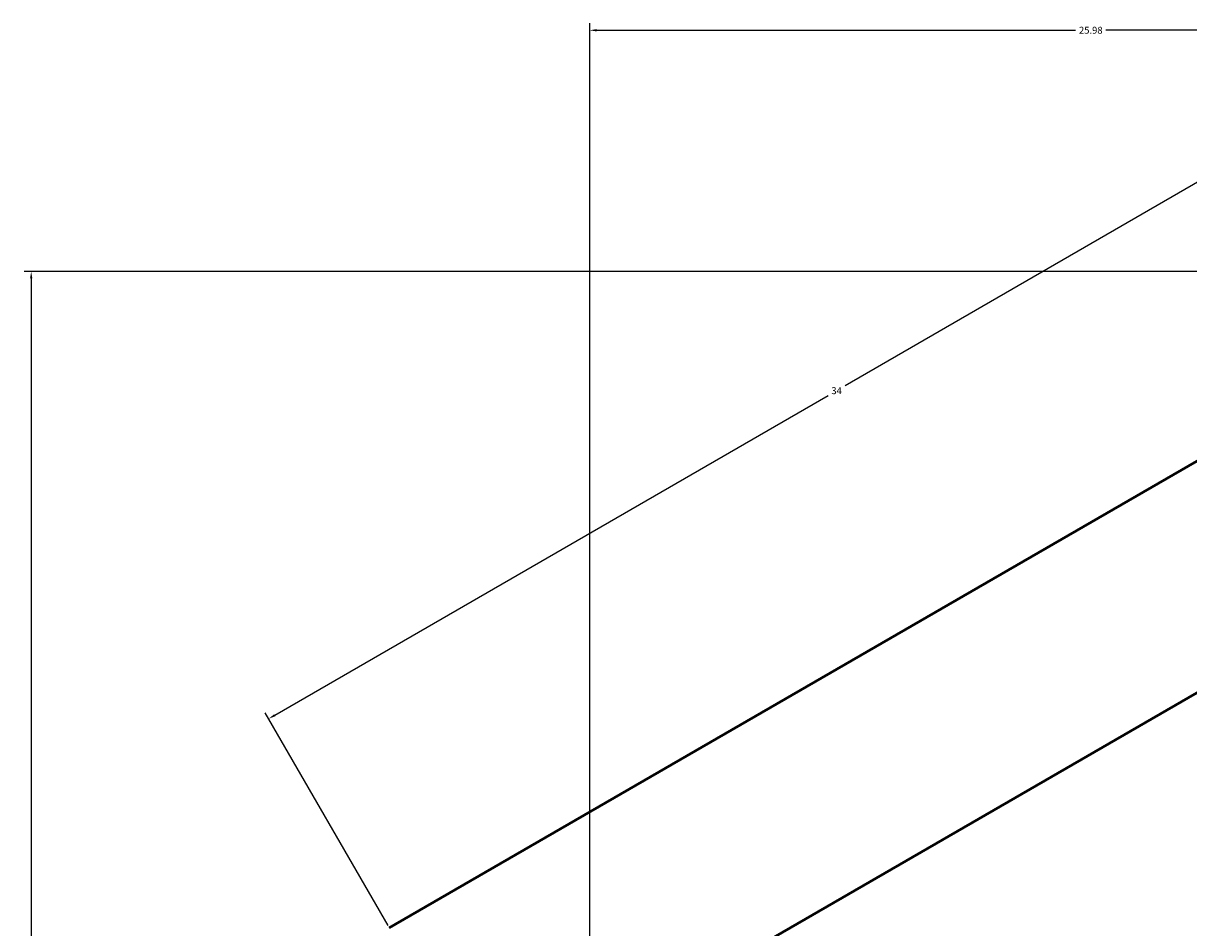
# Model space of a CAD drawing. Units: inches. Extents: x -23 to 69, y -27 to 96.
# Tile 8 of 10: x -23 to 7, y 72 to 96. Entities that reach past the tile are written whole.
import ezdxf

# ---------------------------------------------------------------- set-up
doc = ezdxf.new("R2010")
doc.units = ezdxf.units.IN
doc.header["$MEASUREMENT"] = 0
doc.layers.add('M-DIMS', color=2, linetype='Continuous', lineweight=18)
doc.layers.add('M-OUTL', color=7, linetype='Continuous', lineweight=50)
doc.styles.get("Standard").update_dxf_attribs({"font": 'arial.ttf'})
doc.dimstyles.get("Standard").update_dxf_attribs({"dimtxt": 0.18, "dimasz": 0.18, "dimexe": 0.18, "dimexo": 0.0625, "dimgap": 0.09, "dimtad": 0, "dimtih": 1, "dimtoh": 1, "dimdec": 4, "dimzin": 0, "dimdsep": 46, "dimtxsty": 'Standard', "dimcen": 0.09, "dimadec": 0, "dimazin": 0, "dimtfac": 1, "dimtdec": 4, "dimtofl": 0, "dimtmove": 0, "dimatfit": 3, "dimfxl": 1, "dimtolj": 1, "dimtzin": 0, "dimarcsym": 0})

# ---------------------------------------------------------------- blocks, each defined once
blk = doc.blocks.new('*D8')
at = {"layer": 'Defpoints', "color": 0, "transparency": 16777216}
for p in [(12.713, 94.531), (15.838, 89.119), (-13.607, 72.119)]:
    blk.add_point(p, dxfattribs=at)
at = {"layer": 'M-DIMS', "color": 0, "lineweight": -2, "transparency": 16777216}
for p, q in [((15.807, 89.173), (12.623, 94.687)), ((12.557, 94.441), (-1.791, 86.157)), ((-16.576, 77.621), (-2.228, 85.905)), ((-13.638, 72.173), (-16.822, 77.687))]:
    blk.add_line(p, q, dxfattribs=at)
at = {"layer": 'M-DIMS', "color": 0, "transparency": 16777216}
for points in [[(12.542, 94.467), (12.572, 94.415), (12.713, 94.531)], [(-16.591, 77.647), (-16.561, 77.595), (-16.732, 77.531)]]:
    blk.add_solid(points, dxfattribs=at)
at = {"layer": 'M-DIMS', "color": 0, "transparency": 16777216, "insert": (-2.009, 86.031), "char_height": 0.18, "attachment_point": 5}
blk.add_mtext('\\A1;34', dxfattribs=at)
blk = doc.blocks.new('*D13')
at = {"layer": 'Defpoints', "color": 0, "transparency": 16777216}
for p in [(15.838, 89.119), (-22.888, -20.881), (36.623, -20.881)]:
    blk.add_point(p, dxfattribs=at)
at = {"layer": 'M-DIMS', "color": 0, "lineweight": -2, "transparency": 16777216}
for p, q in [((15.776, 89.119), (-23.068, 89.119)), ((-22.888, 88.939), (-22.888, 34.301)), ((-22.888, -20.701), (-22.888, 33.937)), ((36.56, -20.881), (-23.068, -20.881))]:
    blk.add_line(p, q, dxfattribs=at)
at = {"layer": 'M-DIMS', "color": 0, "transparency": 16777216}
for points in [[(-22.918, 88.939), (-22.858, 88.939), (-22.888, 89.119)], [(-22.918, -20.701), (-22.858, -20.701), (-22.888, -20.881)]]:
    blk.add_solid(points, dxfattribs=at)
at = {"layer": 'M-DIMS', "color": 0, "transparency": 16777216, "insert": (-22.888, 34.119), "char_height": 0.18, "attachment_point": 5}
blk.add_mtext('\\A1;110', dxfattribs=at)
blk = doc.blocks.new('*D16')
at = {"layer": 'Defpoints', "color": 0, "transparency": 16777216}
for p in [(17.57, 95.369), (-8.41, 69.119), (17.57, 52.119)]:
    blk.add_point(p, dxfattribs=at)
at = {"layer": 'M-DIMS', "color": 0, "lineweight": -2, "transparency": 16777216}
for p, q in [((-8.41, 69.181), (-8.41, 95.549)), ((17.57, 52.181), (17.57, 95.549)), ((-8.23, 95.369), (4.184, 95.369)), ((17.39, 95.369), (4.975, 95.369))]:
    blk.add_line(p, q, dxfattribs=at)
at = {"layer": 'M-DIMS', "color": 0, "transparency": 16777216}
for points in [[(-8.23, 95.399), (-8.23, 95.339), (-8.41, 95.369)], [(17.39, 95.399), (17.39, 95.339), (17.57, 95.369)]]:
    blk.add_solid(points, dxfattribs=at)
at = {"layer": 'M-DIMS', "color": 0, "transparency": 16777216, "insert": (4.58, 95.369), "char_height": 0.18, "attachment_point": 5}
blk.add_mtext('\\A1;25.98', dxfattribs=at)

msp = doc.modelspace()

# ---------------------------------------------------------------- linework, layer by layer
at = {"layer": 'M-OUTL'}
for p, q in [((-13.6066, 72.1186), (15.8382, 89.1186)), ((21.0344, 86.1186), (-8.4105, 69.1186))]:
    msp.add_line(p, q, dxfattribs=at)

# ---------------------------------------------------------------- dimensions: what is measured, and where the dimension line sits
at = {"layer": 'M-DIMS'}
dim = msp.add_linear_dim(base=(17.5703, 95.3686), p1=(-8.4105, 69.1186), p2=(17.5703, 52.1186), dimstyle='Standard', override={"dimdec": 2, "dimlfac": 1, "dimrnd": 0, "dimzin": 0, "dimdsep": 46, "dimlunit": 2}, dxfattribs=at)
dim.commit()
dim.dimension.update_dxf_attribs({"geometry": '*D16', "text_midpoint": (4.5799, 95.3686)})
for base, p1, p2, angle, picture, middle in [((12.7132, 94.5313), (-13.6066, 72.1186), (15.8382, 89.1186), 30, '*D8', (-2.0092, 86.0313)), ((-22.8877, -20.8814), (15.8382, 89.1186), (36.6228, -20.8814), 90, '*D13', (-22.8877, 34.1186))]:
    dim = msp.add_linear_dim(base=base, p1=p1, p2=p2, angle=angle, dimstyle='Standard', override={"dimdec": 0, "dimlfac": 1, "dimrnd": 0, "dimzin": 0, "dimdsep": 46, "dimlunit": 2}, dxfattribs=at)
    dim.commit()
    dim.dimension.update_dxf_attribs({"geometry": picture, "text_midpoint": middle})

doc.saveas('drawing.dxf')
